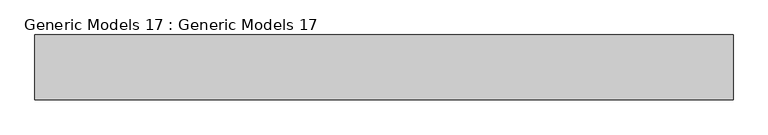
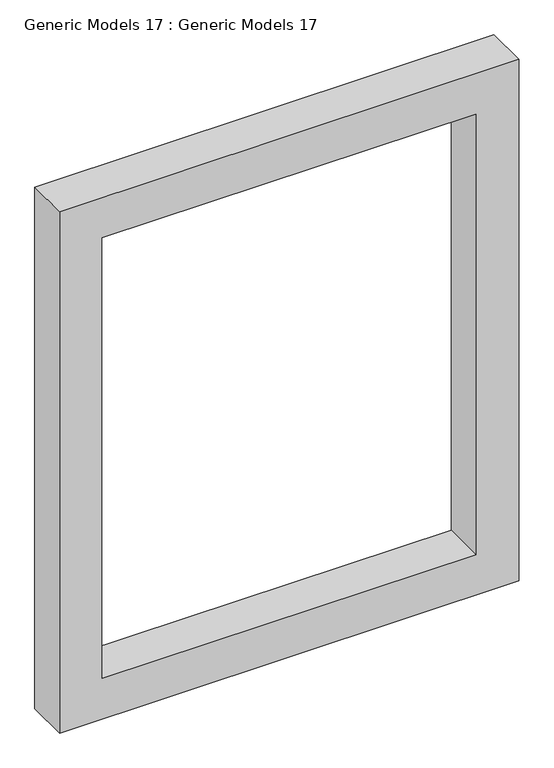
"""IFC4 building model written with IfcOpenShell, lengths in millimetres: proxy geometry, Generic Models 17 : Generic Models 17."""

from ifc_helpers import new_model, si_unit, frame, origin, place, context, project, spatial, polyline, outline, extrude, source, transform, mapped, element, save


def generic_models_17_generic_models_17_71cdcc77(model_context):
    return source(origin(), model_context, "Body", "SweptSolid", [
        extrude(outline(polyline([(2952.75, -10316.1086008), (987.4676291, -10316.1086008), (987.4676291, -8677.8086008), (2952.75, -8677.8086008), (2952.75, -10316.1086008)]), holes=[polyline([(2800.35, -10163.7086008), (2800.35, -8830.2086008), (1139.8676291, -8830.2086008), (1139.8676291, -10163.7086008), (2800.35, -10163.7086008)])]), frame((0.0, 4970.6155883, 0.0), z_axis=(0.0, 1.0, 0.0), x_axis=(0.0, 0.0, 1.0)), (0.0, 0.0, 1.0), 152.4),
    ])


if __name__ == "__main__":
    model = new_model("IFC4")
    model_context = context("Model", 3, world=origin())
    ifc_project = project(units=[si_unit("LENGTHUNIT", "METRE", prefix="MILLI")], contexts=[model_context])
    site = spatial("IfcSite", under=ifc_project)
    building = spatial("IfcBuilding", under=site)
    placement = place(None, origin())
    generic_models_17_generic_models_17_shape = generic_models_17_generic_models_17_71cdcc77(model_context)
    element("IfcBuildingElementProxy", 1, Name="Generic Models 17 : Generic Models 17", ObjectType="Generic Models 17 : Generic Models 17", at=placement, inside=building, context=model_context, shape_type="MappedRepresentation", body=[
        mapped(generic_models_17_generic_models_17_shape, transform((0.0, 0.0, 0.0), x_axis=(1.0, 0.0, 0.0), y_axis=(0.0, 1.0, 0.0), z_axis=(0.0, 0.0, 1.0))),
    ])
    save(model, "model.ifc")

# Revit data of these elements
# Element 1 (IfcBuildingElementProxy, "Generic Models 17 : Generic Models 17")
#   Materials on its faces: "feature frame"
# Materials
#   "feature frame": class "Generic", colour RGB 120 120 120, transparency 0, Cost = 0
